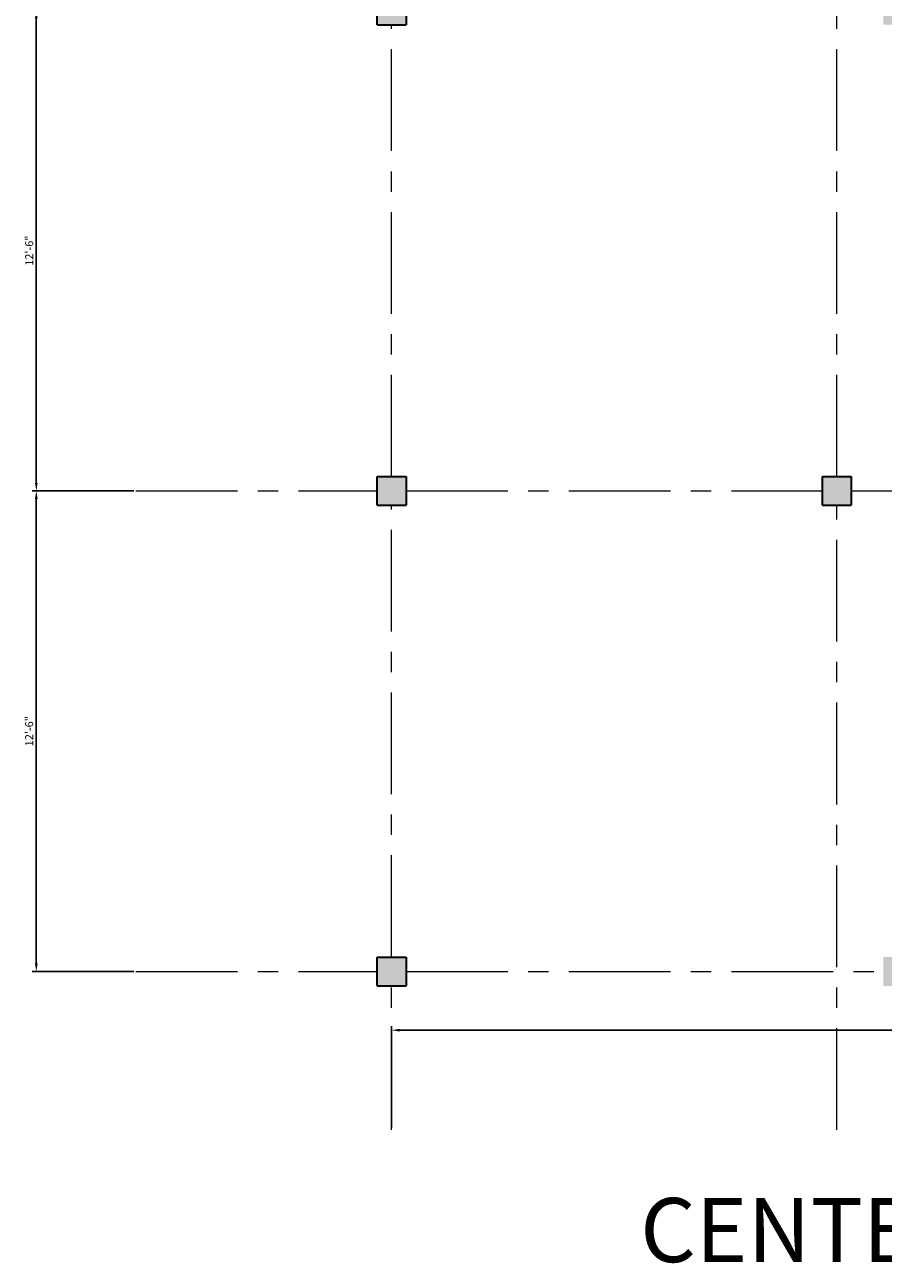
# Model space of a CAD drawing. Units: inches. Extents: x 4878 to 9282, y 5367 to 6617.
# Tile 12 of 14: x 8655 to 8923, y 5977 to 6364. Entities that reach past the tile are written whole.
import ezdxf

# ---------------------------------------------------------------- set-up
doc = ezdxf.new("R2010")
doc.units = ezdxf.units.IN
doc.linetypes.add('CENTER', pattern=[50.8, 31.75, -6.35, 6.35, -6.35])
for name, color, linetype, lineweight in [('A-ANNO-DIMS', 2, 'Continuous', 18), ('A-ANNO-TITL', 3, 'Continuous', 30), ('S-COLS', 1, 'Continuous', 30), ('S-COLS-PATT', 1, 'Continuous', 13), ('S-GRID', 4, 'CENTER', 13)]:
    doc.layers.add(name, color=color, linetype=linetype, lineweight=lineweight)
doc.styles.get("Standard").update_dxf_attribs({"font": 'arial.ttf'})
doc.dimstyles.new('ISO-25', dxfattribs={"dimtxt": 2.5, "dimasz": 2.5, "dimexe": 1.25, "dimexo": 0.625, "dimtad": 1, "dimdec": 0, "dimlunit": 3, "dimtxsty": 'Standard', "dimcen": 2.5, "dimadec": 0, "dimazin": 0, "dimtfac": 1, "dimtdec": 0, "dimtmove": 0, "dimatfit": 3, "dimfxl": 1, "dimarcsym": 0})

# ---------------------------------------------------------------- blocks, each defined once
blk = doc.blocks.new('COLUMN-9X9')
for p, q in [((0, 9), (9, 9)), ((0, 0), (0, 9)), ((9, 9), (9, 0)), ((0, 0), (9, 0))]:
    blk.add_line(p, q)
blk = doc.blocks.new('*D83')
at = {"layer": 'A-ANNO-DIMS', "color": 0, "lineweight": -2, "transparency": 16777216}
for p, q in [((8769.46, 6019.46), (8769.46, 6051.18)), ((9194.46, 6019.46), (9194.46, 6051.18)), ((8771.96, 6049.93), (9191.96, 6049.93))]:
    blk.add_line(p, q, dxfattribs=at)
at = {"layer": 'A-ANNO-DIMS', "color": 0, "transparency": 16777216}
for points in [[(8771.96, 6050.35), (8771.96, 6049.51), (8769.46, 6049.93)], [(9191.96, 6050.35), (9191.96, 6049.51), (9194.46, 6049.93)]]:
    blk.add_solid(points, dxfattribs=at)
at = {"layer": 'Defpoints', "color": 0, "transparency": 16777216}
for p in [(9194.46, 6049.93), (8769.46, 6018.83), (9194.46, 6018.83)]:
    blk.add_point(p, dxfattribs=at)
at = {"layer": 'A-ANNO-DIMS', "color": 0, "transparency": 16777216, "insert": (8981.96, 6051.83), "char_height": 2.5, "attachment_point": 5}
blk.add_mtext('35\'-5"', dxfattribs=at)
blk = doc.blocks.new('*D84')
at = {"layer": 'A-ANNO-DIMS', "color": 0, "lineweight": -2, "transparency": 16777216}
for p, q in [((8688.98, 6218.27), (8657.25, 6218.27)), ((8658.5, 6070.77), (8658.5, 6215.77)), ((8688.98, 6068.27), (8657.25, 6068.27))]:
    blk.add_line(p, q, dxfattribs=at)
at = {"layer": 'A-ANNO-DIMS', "color": 0, "transparency": 16777216}
for points in [[(8658.08, 6215.77), (8658.92, 6215.77), (8658.5, 6218.27)], [(8658.08, 6070.77), (8658.92, 6070.77), (8658.5, 6068.27)]]:
    blk.add_solid(points, dxfattribs=at)
at = {"layer": 'Defpoints', "color": 0, "transparency": 16777216}
for p in [(8658.5, 6218.27), (8689.6, 6218.27), (8689.6, 6068.27)]:
    blk.add_point(p, dxfattribs=at)
at = {"layer": 'A-ANNO-DIMS', "color": 0, "transparency": 16777216, "insert": (8656.6, 6143.27), "char_height": 2.5, "attachment_point": 5, "rotation": 90}
blk.add_mtext('12\'-6"', dxfattribs=at)
blk = doc.blocks.new('*D85')
at = {"layer": 'A-ANNO-DIMS', "color": 0, "lineweight": -2, "transparency": 16777216}
for p, q in [((8688.98, 6368.27), (8657.25, 6368.27)), ((8658.5, 6220.77), (8658.5, 6365.77)), ((8688.98, 6218.27), (8657.25, 6218.27))]:
    blk.add_line(p, q, dxfattribs=at)
at = {"layer": 'A-ANNO-DIMS', "color": 0, "transparency": 16777216}
for points in [[(8658.08, 6365.77), (8658.92, 6365.77), (8658.5, 6368.27)], [(8658.08, 6220.77), (8658.92, 6220.77), (8658.5, 6218.27)]]:
    blk.add_solid(points, dxfattribs=at)
at = {"layer": 'Defpoints', "color": 0, "transparency": 16777216}
for p in [(8658.5, 6368.27), (8689.6, 6368.27), (8689.6, 6218.27)]:
    blk.add_point(p, dxfattribs=at)
at = {"layer": 'A-ANNO-DIMS', "color": 0, "transparency": 16777216, "insert": (8656.6, 6293.27), "char_height": 2.5, "attachment_point": 5, "rotation": 90}
blk.add_mtext('12\'-6"', dxfattribs=at)

msp = doc.modelspace()

# ---------------------------------------------------------------- hatches: boundary and pattern name
at = {"layer": 'S-COLS-PATT'}
h = msp.add_hatch(color=256, dxfattribs=at)
h.dxf.hatch_style = 1
h.paths.add_polyline_path([(8931.96, 6072.77), (8922.96, 6072.77), (8922.96, 6063.77), (8931.96, 6063.77)])
h.paths.add_polyline_path([(9059.96, 6072.77), (9050.96, 6072.77), (9050.96, 6063.77), (9059.96, 6063.77)])
h.paths.add_polyline_path([(9198.96, 6072.77), (9189.96, 6072.77), (9189.96, 6063.77), (9198.96, 6063.77)])
h.paths.add_polyline_path([(9198.96, 6222.77), (9189.96, 6222.77), (9189.96, 6213.77), (9198.96, 6213.77)])
h.paths.add_polyline_path([(9059.96, 6222.77), (9050.96, 6222.77), (9050.96, 6213.77), (9059.96, 6213.77)])
h.paths.add_polyline_path([(8912.96, 6222.77), (8903.96, 6222.77), (8903.96, 6213.77), (8912.96, 6213.77)])
h.paths.add_polyline_path([(8773.96, 6222.77), (8764.96, 6222.77), (8764.96, 6213.77), (8773.96, 6213.77)])
h.paths.add_polyline_path([(8773.96, 6372.77), (8764.96, 6372.77), (8764.96, 6363.77), (8773.96, 6363.77)])
h.paths.add_polyline_path([(8931.96, 6372.77), (8922.96, 6372.77), (8922.96, 6363.77), (8931.96, 6363.77)])
h.paths.add_polyline_path([(9059.96, 6372.77), (9050.96, 6372.77), (9050.96, 6363.77), (9059.96, 6363.77)])
h.paths.add_polyline_path([(9198.96, 6372.77), (9189.96, 6372.77), (9189.96, 6363.77), (9198.96, 6363.77)])
h.paths.add_polyline_path([(9198.96, 6511.77), (9189.96, 6511.77), (9189.96, 6502.77), (9198.96, 6502.77)])
h.paths.add_polyline_path([(9059.96, 6511.77), (9050.96, 6511.77), (9050.96, 6502.77), (9059.96, 6502.77)])
h.paths.add_polyline_path([(8912.96, 6511.77), (8903.96, 6511.77), (8903.96, 6502.77), (8912.96, 6502.77)])
h.paths.add_polyline_path([(8773.96, 6511.77), (8764.96, 6511.77), (8764.96, 6502.77), (8773.96, 6502.77)])
h = msp.add_hatch(color=256, dxfattribs=at)
h.dxf.hatch_style = 1
h.paths.add_polyline_path([(8773.96, 6072.77), (8764.96, 6072.77), (8764.96, 6063.77), (8773.96, 6063.77)])

# ---------------------------------------------------------------- linework, layer by layer
at = {"layer": 'S-COLS'}
msp.add_line((8773.96, 6222.77), (8773.96, 6213.77), dxfattribs=at)
at = {"layer": 'S-GRID'}
for p, q in [((8908.46, 6222.77), (8908.46, 6502.77)), ((8769.46, 6222.77), (8769.46, 6363.77)), ((8689.6, 6218.27), (8764.96, 6218.27)), ((8773.96, 6218.27), (8903.96, 6218.27)), ((8912.96, 6218.27), (9050.96, 6218.27)), ((8769.46, 6072.77), (8769.46, 6213.77)), ((8908.46, 6018.83), (8908.46, 6213.77)), ((8689.6, 6068.27), (8764.96, 6068.27)), ((8773.96, 6068.27), (8922.96, 6068.27)), ((8769.46, 6018.83), (8769.46, 6063.77))]:
    msp.add_line(p, q, dxfattribs=at)

# ---------------------------------------------------------------- block references
at = {"layer": 'S-COLS'}
for p in [(8764.96, 6363.77), (8764.96, 6213.77), (8903.96, 6213.77), (8764.96, 6063.77)]:
    msp.add_blockref('COLUMN-9X9', p, dxfattribs=at)

# ---------------------------------------------------------------- texts
at = {"layer": 'A-ANNO-TITL', "insert": (8847.07, 5997.54), "char_height": 20, "attachment_point": 1}
msp.add_mtext_dynamic_manual_height_columns('CENTER LINE DIAGRAM', width=599.8964, gutter_width=12.5, heights=[0], dxfattribs=at)

# ---------------------------------------------------------------- dimensions: what is measured, and where the dimension line sits
at = {"layer": 'A-ANNO-DIMS'}
for base, p1, p2, picture, middle in [((8658.5, 6368.27), (8689.6, 6218.27), (8689.6, 6368.27), '*D85', (8656.6, 6293.27)), ((8658.5, 6218.27), (8689.6, 6068.27), (8689.6, 6218.27), '*D84', (8656.6, 6143.27))]:
    dim = msp.add_linear_dim(base=base, p1=p1, p2=p2, angle=90, dimstyle='ISO-25', override={"dimdec": 1, "dimlfac": 1, "dimrnd": 0, "dimzin": 1, "dimdsep": 46, "dimlunit": 4, "dimfrac": 2}, dxfattribs=at)
    dim.commit()
    dim.dimension.update_dxf_attribs({"geometry": picture, "text_midpoint": middle})
dim = msp.add_linear_dim(base=(9194.46, 6049.93), p1=(8769.46, 6018.83), p2=(9194.46, 6018.83), dimstyle='ISO-25', override={"dimdec": 1, "dimlfac": 1, "dimrnd": 0, "dimzin": 1, "dimdsep": 46, "dimlunit": 4, "dimfrac": 2}, dxfattribs=at)
dim.commit()
dim.dimension.update_dxf_attribs({"geometry": '*D83', "text_midpoint": (8981.96, 6051.83)})

doc.saveas('drawing.dxf')
